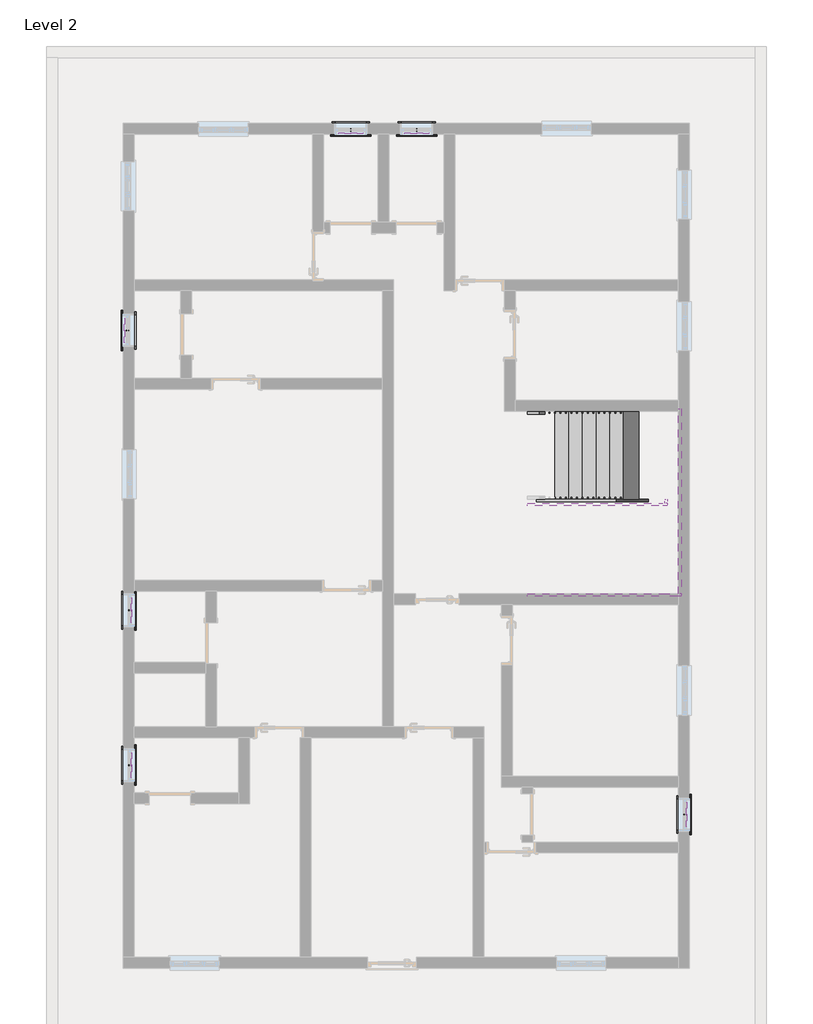
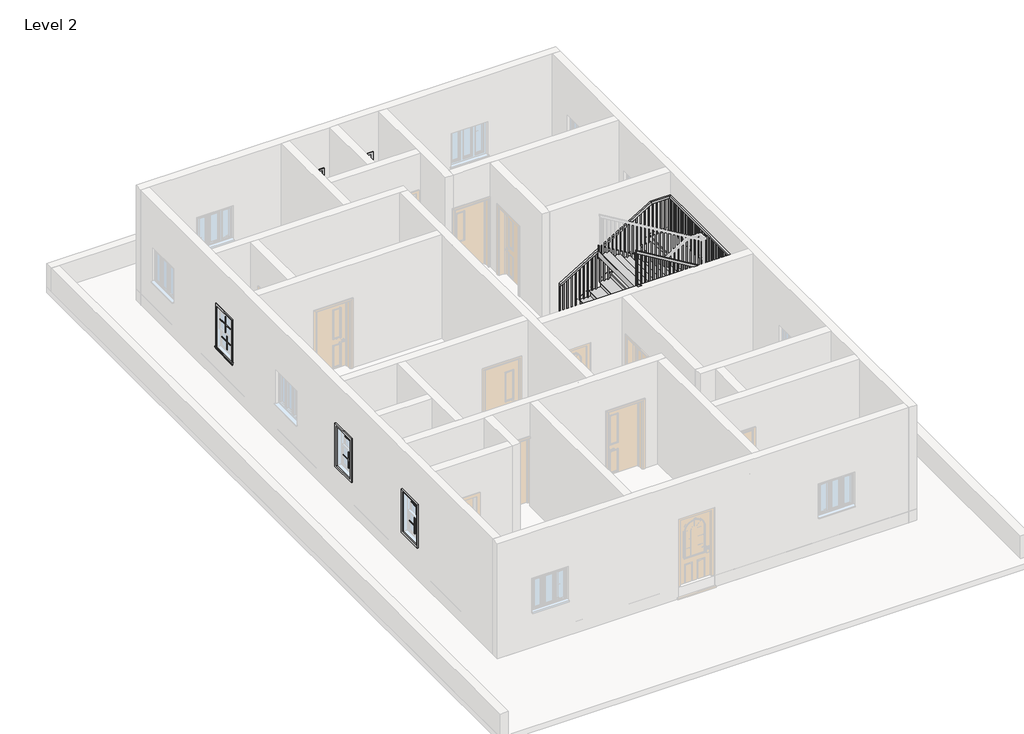
# One storey, part 3 of 3: 24 proxies, 6 members, 1 railing, 1 stair flight.
"""IFC4 building model written with IfcOpenShell, lengths in millimetres."""

from ifc_helpers import new_model, si_unit, frame, origin, place, context, project, spatial, polyline, outline, extrude, faceted_brep, transform, mapped, element, save
from components import muntin_pattern_2x2_muntin_pattern_2x2_eba6c5fb, trim_window_exterior_flat_with_sill_278e6a94, trim_window_interior_flat_picture_frame_e9fd5f45, stair_flight_de280899

model = new_model("IFC4")

# Units and contexts
model_context = context("Model", 3, world=origin())
ifc_project = project(units=[si_unit("LENGTHUNIT", "METRE", prefix="MILLI")], contexts=[model_context])

# Site, building, storey
site = spatial("IfcSite", under=ifc_project)
building = spatial("IfcBuilding", under=site)
storey = spatial("IfcBuildingStorey", under=building, Name="Level 2", Elevation=3048.0)

# Proxies
placement = place(None, origin())
muntin_pattern_2x2_muntin_pattern_2x2_shape = muntin_pattern_2x2_muntin_pattern_2x2_eba6c5fb(model_context)
element("IfcBuildingElementProxy", 1, Name="Muntin Pattern_2x2 : Muntin Pattern_2x2", ObjectType="Muntin Pattern_2x2 : Muntin Pattern_2x2", at=placement, inside=storey, context=model_context, shape_type="MappedRepresentation", body=[
    mapped(muntin_pattern_2x2_muntin_pattern_2x2_shape, transform((-13738.8961241, 8049.5344295, 4518.025), x_axis=(0.0, -1.0, 0.0), y_axis=(1.0, 0.0, 0.0), z_axis=(0.0, 0.0, 1.0))),
])
element("IfcBuildingElementProxy", 2, Name="Muntin Pattern_2x2 : Muntin Pattern_2x2", ObjectType="Muntin Pattern_2x2 : Muntin Pattern_2x2", at=placement, inside=storey, context=model_context, shape_type="MappedRepresentation", body=[
    mapped(muntin_pattern_2x2_muntin_pattern_2x2_shape, transform((-13783.3461241, 8049.5344295, 4038.6), x_axis=(0.0, -1.0, 0.0), y_axis=(1.0, 0.0, 0.0), z_axis=(0.0, 0.0, 1.0))),
])
element("IfcBuildingElementProxy", 3, Name="Muntin Pattern_2x2 : Muntin Pattern_2x2", ObjectType="Muntin Pattern_2x2 : Muntin Pattern_2x2", at=placement, inside=storey, context=model_context, shape_type="MappedRepresentation", body=[
    mapped(muntin_pattern_2x2_muntin_pattern_2x2_shape, transform((-13738.8961241, 5179.3344295, 4518.025), x_axis=(0.0, -1.0, 0.0), y_axis=(1.0, 0.0, 0.0), z_axis=(0.0, 0.0, 1.0))),
])
element("IfcBuildingElementProxy", 4, Name="Muntin Pattern_2x2 : Muntin Pattern_2x2", ObjectType="Muntin Pattern_2x2 : Muntin Pattern_2x2", at=placement, inside=storey, context=model_context, shape_type="MappedRepresentation", body=[
    mapped(muntin_pattern_2x2_muntin_pattern_2x2_shape, transform((-13783.3461241, 5179.3344295, 4038.6), x_axis=(0.0, -1.0, 0.0), y_axis=(1.0, 0.0, 0.0), z_axis=(0.0, 0.0, 1.0))),
])
element("IfcBuildingElementProxy", 5, Name="Muntin Pattern_2x2 : Muntin Pattern_2x2", ObjectType="Muntin Pattern_2x2 : Muntin Pattern_2x2", at=placement, inside=storey, context=model_context, shape_type="MappedRepresentation", body=[
    mapped(muntin_pattern_2x2_muntin_pattern_2x2_shape, transform((-13872.2461241, 13231.1344295, 4518.025), x_axis=(0.0, 1.0, 0.0), y_axis=(-1.0, 0.0, 0.0), z_axis=(0.0, 0.0, 1.0))),
])
element("IfcBuildingElementProxy", 6, Name="Muntin Pattern_2x2 : Muntin Pattern_2x2", ObjectType="Muntin Pattern_2x2 : Muntin Pattern_2x2", at=placement, inside=storey, context=model_context, shape_type="MappedRepresentation", body=[
    mapped(muntin_pattern_2x2_muntin_pattern_2x2_shape, transform((-13827.7961241, 13231.1344295, 4038.6), x_axis=(0.0, 1.0, 0.0), y_axis=(-1.0, 0.0, 0.0), z_axis=(0.0, 0.0, 1.0))),
])
element("IfcBuildingElementProxy", 7, Name="Muntin Pattern_2x2 : Muntin Pattern_2x2", ObjectType="Muntin Pattern_2x2 : Muntin Pattern_2x2", at=placement, inside=storey, context=model_context, shape_type="MappedRepresentation", body=[
    mapped(muntin_pattern_2x2_muntin_pattern_2x2_shape, transform((-9690.7711241, 16898.2594295, 4518.025), x_axis=(-1.0, 0.0, 0.0), y_axis=(0.0, -1.0, 0.0), z_axis=(0.0, 0.0, 1.0))),
])
element("IfcBuildingElementProxy", 8, Name="Muntin Pattern_2x2 : Muntin Pattern_2x2", ObjectType="Muntin Pattern_2x2 : Muntin Pattern_2x2", at=placement, inside=storey, context=model_context, shape_type="MappedRepresentation", body=[
    mapped(muntin_pattern_2x2_muntin_pattern_2x2_shape, transform((-9690.7711241, 16942.7094295, 4038.6), x_axis=(-1.0, 0.0, 0.0), y_axis=(0.0, -1.0, 0.0), z_axis=(0.0, 0.0, 1.0))),
])
element("IfcBuildingElementProxy", 9, Name="Muntin Pattern_2x2 : Muntin Pattern_2x2", ObjectType="Muntin Pattern_2x2 : Muntin Pattern_2x2", at=placement, inside=storey, context=model_context, shape_type="MappedRepresentation", body=[
    mapped(muntin_pattern_2x2_muntin_pattern_2x2_shape, transform((-8471.5711241, 16898.2594295, 4518.025), x_axis=(-1.0, 0.0, 0.0), y_axis=(0.0, -1.0, 0.0), z_axis=(0.0, 0.0, 1.0))),
])
element("IfcBuildingElementProxy", 10, Name="Muntin Pattern_2x2 : Muntin Pattern_2x2", ObjectType="Muntin Pattern_2x2 : Muntin Pattern_2x2", at=placement, inside=storey, context=model_context, shape_type="MappedRepresentation", body=[
    mapped(muntin_pattern_2x2_muntin_pattern_2x2_shape, transform((-8471.5711241, 16942.7094295, 4038.6), x_axis=(-1.0, 0.0, 0.0), y_axis=(0.0, -1.0, 0.0), z_axis=(0.0, 0.0, 1.0))),
])
element("IfcBuildingElementProxy", 11, Name="Muntin Pattern_2x2 : Muntin Pattern_2x2", ObjectType="Muntin Pattern_2x2 : Muntin Pattern_2x2", at=placement, inside=storey, context=model_context, shape_type="MappedRepresentation", body=[
    mapped(muntin_pattern_2x2_muntin_pattern_2x2_shape, transform((-3451.8961241, 4264.9344295, 4518.025), x_axis=(0.0, -1.0, 0.0), y_axis=(1.0, 0.0, 0.0), z_axis=(0.0, 0.0, 1.0))),
])
element("IfcBuildingElementProxy", 12, Name="Muntin Pattern_2x2 : Muntin Pattern_2x2", ObjectType="Muntin Pattern_2x2 : Muntin Pattern_2x2", at=placement, inside=storey, context=model_context, shape_type="MappedRepresentation", body=[
    mapped(muntin_pattern_2x2_muntin_pattern_2x2_shape, transform((-3496.3461241, 4264.9344295, 4038.6), x_axis=(0.0, -1.0, 0.0), y_axis=(1.0, 0.0, 0.0), z_axis=(0.0, 0.0, 1.0))),
])
trim_window_exterior_flat_with_sill_shape = trim_window_exterior_flat_with_sill_278e6a94(model_context)
element("IfcBuildingElementProxy", 13, Name="Trim-Window-Exterior-Flat : with Sill", ObjectType="Trim-Window-Exterior-Flat : with Sill", at=placement, inside=storey, context=model_context, shape_type="MappedRepresentation", body=[
    mapped(trim_window_exterior_flat_with_sill_shape, transform((-13703.9711241, 8049.5344295, 5029.2), x_axis=(0.0, 1.0, 0.0), y_axis=(0.0, 0.0, 1.0), z_axis=(1.0, 0.0, 0.0))),
])
element("IfcBuildingElementProxy", 14, Name="Trim-Window-Exterior-Flat : with Sill", ObjectType="Trim-Window-Exterior-Flat : with Sill", at=placement, inside=storey, context=model_context, shape_type="MappedRepresentation", body=[
    mapped(trim_window_exterior_flat_with_sill_shape, transform((-13703.9711241, 5179.3344295, 5029.2), x_axis=(0.0, 1.0, 0.0), y_axis=(0.0, 0.0, 1.0), z_axis=(1.0, 0.0, 0.0))),
])
element("IfcBuildingElementProxy", 15, Name="Trim-Window-Exterior-Flat : with Sill", ObjectType="Trim-Window-Exterior-Flat : with Sill", at=placement, inside=storey, context=model_context, shape_type="MappedRepresentation", body=[
    mapped(trim_window_exterior_flat_with_sill_shape, transform((-13907.1711241, 13231.1344295, 5029.2), x_axis=(0.0, -1.0, 0.0), y_axis=(0.0, 0.0, 1.0), z_axis=(-1.0, 0.0, 0.0))),
])
element("IfcBuildingElementProxy", 16, Name="Trim-Window-Exterior-Flat : with Sill", ObjectType="Trim-Window-Exterior-Flat : with Sill", at=placement, inside=storey, context=model_context, shape_type="MappedRepresentation", body=[
    mapped(trim_window_exterior_flat_with_sill_shape, transform((-9690.7711241, 16863.3344295, 5029.2), x_axis=(1.0, 0.0, 0.0), y_axis=(0.0, 0.0, 1.0), z_axis=(0.0, -1.0, 0.0))),
])
element("IfcBuildingElementProxy", 17, Name="Trim-Window-Exterior-Flat : with Sill", ObjectType="Trim-Window-Exterior-Flat : with Sill", at=placement, inside=storey, context=model_context, shape_type="MappedRepresentation", body=[
    mapped(trim_window_exterior_flat_with_sill_shape, transform((-8471.5711241, 16863.3344295, 5029.2), x_axis=(1.0, 0.0, 0.0), y_axis=(0.0, 0.0, 1.0), z_axis=(0.0, -1.0, 0.0))),
])
element("IfcBuildingElementProxy", 18, Name="Trim-Window-Exterior-Flat : with Sill", ObjectType="Trim-Window-Exterior-Flat : with Sill", at=placement, inside=storey, context=model_context, shape_type="MappedRepresentation", body=[
    mapped(trim_window_exterior_flat_with_sill_shape, transform((-3416.9711241, 4264.9344295, 5029.2), x_axis=(0.0, 1.0, 0.0), y_axis=(0.0, 0.0, 1.0), z_axis=(1.0, 0.0, 0.0))),
])
trim_window_interior_flat_picture_frame_shape = trim_window_interior_flat_picture_frame_e9fd5f45(model_context)
element("IfcBuildingElementProxy", 19, Name="Trim-Window-Interior-Flat : Picture Frame", ObjectType="Trim-Window-Interior-Flat : Picture Frame", at=placement, inside=storey, context=model_context, shape_type="MappedRepresentation", body=[
    mapped(trim_window_interior_flat_picture_frame_shape, transform((-13907.1711241, 8049.5344295, 5029.2), x_axis=(0.0, -1.0, 0.0), y_axis=(0.0, 0.0, 1.0), z_axis=(-1.0, 0.0, 0.0))),
])
element("IfcBuildingElementProxy", 20, Name="Trim-Window-Interior-Flat : Picture Frame", ObjectType="Trim-Window-Interior-Flat : Picture Frame", at=placement, inside=storey, context=model_context, shape_type="MappedRepresentation", body=[
    mapped(trim_window_interior_flat_picture_frame_shape, transform((-13907.1711241, 5179.3344295, 5029.2), x_axis=(0.0, -1.0, 0.0), y_axis=(0.0, 0.0, 1.0), z_axis=(-1.0, 0.0, 0.0))),
])
element("IfcBuildingElementProxy", 21, Name="Trim-Window-Interior-Flat : Picture Frame", ObjectType="Trim-Window-Interior-Flat : Picture Frame", at=placement, inside=storey, context=model_context, shape_type="MappedRepresentation", body=[
    mapped(trim_window_interior_flat_picture_frame_shape, transform((-13703.9711241, 13231.1344295, 5029.2), x_axis=(0.0, 1.0, 0.0), y_axis=(0.0, 0.0, 1.0), z_axis=(1.0, 0.0, 0.0))),
])
element("IfcBuildingElementProxy", 22, Name="Trim-Window-Interior-Flat : Picture Frame", ObjectType="Trim-Window-Interior-Flat : Picture Frame", at=placement, inside=storey, context=model_context, shape_type="MappedRepresentation", body=[
    mapped(trim_window_interior_flat_picture_frame_shape, transform((-9690.7711241, 17066.5344295, 5029.2), x_axis=(-1.0, 0.0, 0.0), y_axis=(0.0, 0.0, 1.0), z_axis=(0.0, 1.0, 0.0))),
])
element("IfcBuildingElementProxy", 23, Name="Trim-Window-Interior-Flat : Picture Frame", ObjectType="Trim-Window-Interior-Flat : Picture Frame", at=placement, inside=storey, context=model_context, shape_type="MappedRepresentation", body=[
    mapped(trim_window_interior_flat_picture_frame_shape, transform((-8471.5711241, 17066.5344295, 5029.2), x_axis=(-1.0, 0.0, 0.0), y_axis=(0.0, 0.0, 1.0), z_axis=(0.0, 1.0, 0.0))),
])
element("IfcBuildingElementProxy", 24, Name="Trim-Window-Interior-Flat : Picture Frame", ObjectType="Trim-Window-Interior-Flat : Picture Frame", at=placement, inside=storey, context=model_context, shape_type="MappedRepresentation", body=[
    mapped(trim_window_interior_flat_picture_frame_shape, transform((-3620.1711241, 4264.9344295, 5029.2), x_axis=(0.0, -1.0, 0.0), y_axis=(0.0, 0.0, 1.0), z_axis=(-1.0, 0.0, 0.0))),
])

# Members
element("IfcMember", 25, ObjectType="Stringer - 2\" Width", at=placement, inside=storey, context=model_context, shape_type="SweptSolid", body=[
    extrude(outline(polyline([(3259.5517384, -6414.1711241), (3048.0, -6414.1711241), (3048.0, -6174.3326423), (4580.4969109, -3620.1711241), (4648.2, -3620.1711241), (4648.2, -4099.7573548), (3259.5517384, -6414.1711241)])), frame((0.0, 11732.5344295, 0.0), z_axis=(0.0, 1.0, 0.0), x_axis=(0.0, 0.0, 1.0)), (0.0, 0.0, 1.0), 50.8),
])
element("IfcMember", 26, ObjectType="Stringer - 2\" Width", at=placement, inside=storey, context=model_context, shape_type="SweptSolid", body=[
    extrude(outline(polyline([(-3620.1711241, 11783.3344295), (-3569.3711241, 11783.3344295), (-3569.3711241, 8354.3344295), (-3620.1711241, 8354.3344295), (-3620.1711241, 11783.3344295)])), frame((0.0, 0.0, 4343.4), z_axis=(0.0, 0.0, 1.0), x_axis=(1.0, 0.0, 0.0)), (0.0, 0.0, 1.0), 304.8),
])
element("IfcMember", 27, ObjectType="Stringer - 2\" Width", at=placement, inside=storey, context=model_context, shape_type="SweptSolid", body=[
    extrude(outline(polyline([(4343.4, -3569.3711241), (4448.2717384, -3569.3711241), (6155.1517384, -6414.1711241), (5799.6969109, -6414.1711241), (4343.4, -3987.0096058), (4343.4, -3569.3711241)])), frame((0.0, 8303.5344295, 0.0), z_axis=(0.0, 1.0, 0.0), x_axis=(0.0, 0.0, 1.0)), (0.0, 0.0, 1.0), 50.8),
])
element("IfcMember", 28, ObjectType="Stringer - 2\" Width", at=placement, inside=storey, context=model_context, shape_type="SweptSolid", body=[
    extrude(outline(polyline([(3259.5517384, -6414.1711241), (3048.0, -6414.1711241), (3048.0, -6174.3326423), (4428.0969109, -3874.1711241), (4648.2, -3874.1711241), (4648.2, -4099.7573548), (3259.5517384, -6414.1711241)])), frame((0.0, 10056.1344295, 0.0), z_axis=(0.0, 1.0, 0.0), x_axis=(0.0, 0.0, 1.0)), (0.0, 0.0, 1.0), 50.8),
])
element("IfcMember", 29, ObjectType="Stringer - 2\" Width", at=placement, inside=storey, context=model_context, shape_type="SweptSolid", body=[
    extrude(outline(polyline([(-3874.1711241, 10106.9344295), (-3823.3711241, 10106.9344295), (-3823.3711241, 10030.7344295), (-3874.1711241, 10030.7344295), (-3874.1711241, 10106.9344295)])), frame((0.0, 0.0, 4343.4), z_axis=(0.0, 0.0, 1.0), x_axis=(1.0, 0.0, 0.0)), (0.0, 0.0, 1.0), 304.8),
])
element("IfcMember", 30, ObjectType="Stringer - 2\" Width", at=placement, inside=storey, context=model_context, shape_type="SweptSolid", body=[
    extrude(outline(polyline([(4343.4, -3823.3711241), (4600.6717384, -3823.3711241), (6155.1517384, -6414.1711241), (5799.6969109, -6414.1711241), (4343.4, -3987.0096058), (4343.4, -3823.3711241)])), frame((0.0, 9979.9344295, 0.0), z_axis=(0.0, 1.0, 0.0), x_axis=(0.0, 0.0, 1.0)), (0.0, 0.0, 1.0), 50.8),
])

# Railing
element("IfcRailing", 31, ObjectType="Handrail - Rectangular", at=placement, inside=storey, context=model_context, shape_type="SolidModel", body=[
    faceted_brep([(-6414.1711241, 11732.5344295, 4114.8), (-6414.1711241, 11732.5344295, 4055.5575287), (-6414.1711241, 11681.7344295, 4055.5575287), (-6414.1711241, 11681.7344295, 4114.8), (-4128.1711241, 11732.5344295, 5486.4), (-4114.1003386, 11732.5344295, 5435.6), (-4114.1003386, 11681.7344295, 5435.6), (-4128.1711241, 11681.7344295, 5486.4), (-3620.1711241, 11732.5344295, 5486.4), (-3620.1711241, 11732.5344295, 5435.6), (-3670.9711241, 11681.7344295, 5435.6), (-3670.9711241, 11681.7344295, 5486.4), (-3620.1711241, 8354.3344295, 5486.4), (-3620.1711241, 8354.3344295, 5435.6), (-3670.9711241, 8405.1344295, 5435.6), (-3670.9711241, 8405.1344295, 5486.4), (-3874.1711241, 8354.3344295, 5486.4), (-3888.2419095, 8354.3344295, 5435.6), (-3888.2419095, 8405.1344295, 5435.6), (-3874.1711241, 8405.1344295, 5486.4), (-6414.1711241, 8354.3344295, 7010.4), (-6414.1711241, 8405.1344295, 7010.4), (-6414.1711241, 8405.1344295, 6951.1575287), (-6414.1711241, 8354.3344295, 6951.1575287)], [[[0, 1, 2, 3]], [[1, 0, 4, 5]], [[2, 1, 5, 6]], [[3, 2, 6, 7]], [[0, 3, 7, 4]], [[5, 4, 8, 9]], [[6, 5, 9, 10]], [[7, 6, 10, 11]], [[4, 7, 11, 8]], [[9, 8, 12, 13]], [[10, 9, 13, 14]], [[11, 10, 14, 15]], [[8, 11, 15, 12]], [[13, 12, 16, 17]], [[14, 13, 17, 18]], [[15, 14, 18, 19]], [[12, 15, 19, 16]], [[20, 21, 22, 23]], [[17, 16, 20, 23]], [[18, 17, 23, 22]], [[19, 18, 22, 21]], [[16, 19, 21, 20]]]),
    extrude(outline(polyline([(6941.6325287, -6398.2961241), (5943.6, -6398.2961241), (5943.6, -6379.2461241), (6930.2025287, -6379.2461241), (6941.6325287, -6398.2961241)])), frame((0.0, 8370.2094295, 0.0), z_axis=(0.0, 1.0, 0.0), x_axis=(0.0, 0.0, 1.0)), (0.0, 0.0, 1.0), 19.05),
    extrude(outline(polyline([(6880.6725287, -6296.6961241), (5943.6, -6296.6961241), (5943.6, -6277.6461241), (6869.2425287, -6277.6461241), (6880.6725287, -6296.6961241)])), frame((0.0, 8370.2094295, 0.0), z_axis=(0.0, 1.0, 0.0), x_axis=(0.0, 0.0, 1.0)), (0.0, 0.0, 1.0), 19.05),
    extrude(outline(polyline([(6819.7125287, -6195.0961241), (5943.6, -6195.0961241), (5943.6, -6176.0461241), (6808.2825287, -6176.0461241), (6819.7125287, -6195.0961241)])), frame((0.0, 8370.2094295, 0.0), z_axis=(0.0, 1.0, 0.0), x_axis=(0.0, 0.0, 1.0)), (0.0, 0.0, 1.0), 19.05),
    extrude(outline(polyline([(6758.7525287, -6093.4961241), (5791.2, -6093.4961241), (5791.2, -6074.4461241), (6747.3225287, -6074.4461241), (6758.7525287, -6093.4961241)])), frame((0.0, 8370.2094295, 0.0), z_axis=(0.0, 1.0, 0.0), x_axis=(0.0, 0.0, 1.0)), (0.0, 0.0, 1.0), 19.05),
    extrude(outline(polyline([(6697.7925287, -5991.8961241), (5791.2, -5991.8961241), (5791.2, -5972.8461241), (6686.3625287, -5972.8461241), (6697.7925287, -5991.8961241)])), frame((0.0, 8370.2094295, 0.0), z_axis=(0.0, 1.0, 0.0), x_axis=(0.0, 0.0, 1.0)), (0.0, 0.0, 1.0), 19.05),
    extrude(outline(polyline([(6636.8325287, -5890.2961241), (5638.8, -5890.2961241), (5638.8, -5871.2461241), (6625.4025287, -5871.2461241), (6636.8325287, -5890.2961241)])), frame((0.0, 8370.2094295, 0.0), z_axis=(0.0, 1.0, 0.0), x_axis=(0.0, 0.0, 1.0)), (0.0, 0.0, 1.0), 19.05),
    extrude(outline(polyline([(6575.8725287, -5788.6961241), (5638.8, -5788.6961241), (5638.8, -5769.6461241), (6564.4425287, -5769.6461241), (6575.8725287, -5788.6961241)])), frame((0.0, 8370.2094295, 0.0), z_axis=(0.0, 1.0, 0.0), x_axis=(0.0, 0.0, 1.0)), (0.0, 0.0, 1.0), 19.05),
    extrude(outline(polyline([(6514.9125287, -5687.0961241), (5638.8, -5687.0961241), (5638.8, -5668.0461241), (6503.4825287, -5668.0461241), (6514.9125287, -5687.0961241)])), frame((0.0, 8370.2094295, 0.0), z_axis=(0.0, 1.0, 0.0), x_axis=(0.0, 0.0, 1.0)), (0.0, 0.0, 1.0), 19.05),
    extrude(outline(polyline([(6453.9525287, -5585.4961241), (5486.4, -5585.4961241), (5486.4, -5566.4461241), (6442.5225287, -5566.4461241), (6453.9525287, -5585.4961241)])), frame((0.0, 8370.2094295, 0.0), z_axis=(0.0, 1.0, 0.0), x_axis=(0.0, 0.0, 1.0)), (0.0, 0.0, 1.0), 19.05),
    extrude(outline(polyline([(6392.9925287, -5483.8961241), (5486.4, -5483.8961241), (5486.4, -5464.8461241), (6381.5625287, -5464.8461241), (6392.9925287, -5483.8961241)])), frame((0.0, 8370.2094295, 0.0), z_axis=(0.0, 1.0, 0.0), x_axis=(0.0, 0.0, 1.0)), (0.0, 0.0, 1.0), 19.05),
    extrude(outline(polyline([(6332.0325287, -5382.2961241), (5334.0, -5382.2961241), (5334.0, -5363.2461241), (6320.6025287, -5363.2461241), (6332.0325287, -5382.2961241)])), frame((0.0, 8370.2094295, 0.0), z_axis=(0.0, 1.0, 0.0), x_axis=(0.0, 0.0, 1.0)), (0.0, 0.0, 1.0), 19.05),
    extrude(outline(polyline([(6271.0725287, -5280.6961241), (5334.0, -5280.6961241), (5334.0, -5261.6461241), (6259.6425287, -5261.6461241), (6271.0725287, -5280.6961241)])), frame((0.0, 8370.2094295, 0.0), z_axis=(0.0, 1.0, 0.0), x_axis=(0.0, 0.0, 1.0)), (0.0, 0.0, 1.0), 19.05),
    extrude(outline(polyline([(6210.1125287, -5179.0961241), (5334.0, -5179.0961241), (5334.0, -5160.0461241), (6198.6825287, -5160.0461241), (6210.1125287, -5179.0961241)])), frame((0.0, 8370.2094295, 0.0), z_axis=(0.0, 1.0, 0.0), x_axis=(0.0, 0.0, 1.0)), (0.0, 0.0, 1.0), 19.05),
    extrude(outline(polyline([(6149.1525287, -5077.4961241), (5181.6, -5077.4961241), (5181.6, -5058.4461241), (6137.7225287, -5058.4461241), (6149.1525287, -5077.4961241)])), frame((0.0, 8370.2094295, 0.0), z_axis=(0.0, 1.0, 0.0), x_axis=(0.0, 0.0, 1.0)), (0.0, 0.0, 1.0), 19.05),
    extrude(outline(polyline([(6088.1925287, -4975.8961241), (5181.6, -4975.8961241), (5181.6, -4956.8461241), (6076.7625287, -4956.8461241), (6088.1925287, -4975.8961241)])), frame((0.0, 8370.2094295, 0.0), z_axis=(0.0, 1.0, 0.0), x_axis=(0.0, 0.0, 1.0)), (0.0, 0.0, 1.0), 19.05),
    extrude(outline(polyline([(6027.2325287, -4874.2961241), (5029.2, -4874.2961241), (5029.2, -4855.2461241), (6015.8025287, -4855.2461241), (6027.2325287, -4874.2961241)])), frame((0.0, 8370.2094295, 0.0), z_axis=(0.0, 1.0, 0.0), x_axis=(0.0, 0.0, 1.0)), (0.0, 0.0, 1.0), 19.05),
    extrude(outline(polyline([(5966.2725287, -4772.6961241), (5029.2, -4772.6961241), (5029.2, -4753.6461241), (5954.8425287, -4753.6461241), (5966.2725287, -4772.6961241)])), frame((0.0, 8370.2094295, 0.0), z_axis=(0.0, 1.0, 0.0), x_axis=(0.0, 0.0, 1.0)), (0.0, 0.0, 1.0), 19.05),
    extrude(outline(polyline([(5905.3125287, -4671.0961241), (5029.2, -4671.0961241), (5029.2, -4652.0461241), (5893.8825287, -4652.0461241), (5905.3125287, -4671.0961241)])), frame((0.0, 8370.2094295, 0.0), z_axis=(0.0, 1.0, 0.0), x_axis=(0.0, 0.0, 1.0)), (0.0, 0.0, 1.0), 19.05),
    extrude(outline(polyline([(5844.3525287, -4569.4961241), (4876.8, -4569.4961241), (4876.8, -4550.4461241), (5832.9225287, -4550.4461241), (5844.3525287, -4569.4961241)])), frame((0.0, 8370.2094295, 0.0), z_axis=(0.0, 1.0, 0.0), x_axis=(0.0, 0.0, 1.0)), (0.0, 0.0, 1.0), 19.05),
    extrude(outline(polyline([(5783.3925287, -4467.8961241), (4876.8, -4467.8961241), (4876.8, -4448.8461241), (5771.9625287, -4448.8461241), (5783.3925287, -4467.8961241)])), frame((0.0, 8370.2094295, 0.0), z_axis=(0.0, 1.0, 0.0), x_axis=(0.0, 0.0, 1.0)), (0.0, 0.0, 1.0), 19.05),
    extrude(outline(polyline([(5722.4325287, -4366.2961241), (4724.4, -4366.2961241), (4724.4, -4347.2461241), (5711.0025287, -4347.2461241), (5722.4325287, -4366.2961241)])), frame((0.0, 8370.2094295, 0.0), z_axis=(0.0, 1.0, 0.0), x_axis=(0.0, 0.0, 1.0)), (0.0, 0.0, 1.0), 19.05),
    extrude(outline(polyline([(5661.4725287, -4264.6961241), (4724.4, -4264.6961241), (4724.4, -4245.6461241), (5650.0425287, -4245.6461241), (5661.4725287, -4264.6961241)])), frame((0.0, 8370.2094295, 0.0), z_axis=(0.0, 1.0, 0.0), x_axis=(0.0, 0.0, 1.0)), (0.0, 0.0, 1.0), 19.05),
    extrude(outline(polyline([(5600.5125287, -4163.0961241), (4724.4, -4163.0961241), (4724.4, -4144.0461241), (5589.0825287, -4144.0461241), (5600.5125287, -4163.0961241)])), frame((0.0, 8370.2094295, 0.0), z_axis=(0.0, 1.0, 0.0), x_axis=(0.0, 0.0, 1.0)), (0.0, 0.0, 1.0), 19.05),
    extrude(outline(polyline([(5539.5525287, -4061.4961241), (4572.0, -4061.4961241), (4572.0, -4042.4461241), (5528.1225287, -4042.4461241), (5539.5525287, -4061.4961241)])), frame((0.0, 8370.2094295, 0.0), z_axis=(0.0, 1.0, 0.0), x_axis=(0.0, 0.0, 1.0)), (0.0, 0.0, 1.0), 19.05),
    extrude(outline(polyline([(5478.5925287, -3959.8961241), (4572.0, -3959.8961241), (4572.0, -3940.8461241), (5467.1625287, -3940.8461241), (5478.5925287, -3959.8961241)])), frame((0.0, 8370.2094295, 0.0), z_axis=(0.0, 1.0, 0.0), x_axis=(0.0, 0.0, 1.0)), (0.0, 0.0, 1.0), 19.05),
    extrude(outline(polyline([(-3839.2461241, 8370.2094295), (-3858.2961241, 8370.2094295), (-3858.2961241, 8389.2594295), (-3839.2461241, 8389.2594295), (-3839.2461241, 8370.2094295)])), frame((0.0, 0.0, 4572.0), z_axis=(0.0, 0.0, 1.0), x_axis=(1.0, 0.0, 0.0)), (0.0, 0.0, 1.0), 863.6),
    extrude(outline(polyline([(-3737.6461241, 8370.2094295), (-3756.6961241, 8370.2094295), (-3756.6961241, 8389.2594295), (-3737.6461241, 8389.2594295), (-3737.6461241, 8370.2094295)])), frame((0.0, 0.0, 4572.0), z_axis=(0.0, 0.0, 1.0), x_axis=(1.0, 0.0, 0.0)), (0.0, 0.0, 1.0), 863.6),
    extrude(outline(polyline([(-3636.0461241, 8465.4594295), (-3636.0461241, 8446.4094295), (-3655.0961241, 8446.4094295), (-3655.0961241, 8465.4594295), (-3636.0461241, 8465.4594295)])), frame((0.0, 0.0, 4572.0), z_axis=(0.0, 0.0, 1.0), x_axis=(1.0, 0.0, 0.0)), (0.0, 0.0, 1.0), 863.6),
    extrude(outline(polyline([(-3636.0461241, 8567.0594295), (-3636.0461241, 8548.0094295), (-3655.0961241, 8548.0094295), (-3655.0961241, 8567.0594295), (-3636.0461241, 8567.0594295)])), frame((0.0, 0.0, 4572.0), z_axis=(0.0, 0.0, 1.0), x_axis=(1.0, 0.0, 0.0)), (0.0, 0.0, 1.0), 863.6),
    extrude(outline(polyline([(-3636.0461241, 8668.6594295), (-3636.0461241, 8649.6094295), (-3655.0961241, 8649.6094295), (-3655.0961241, 8668.6594295), (-3636.0461241, 8668.6594295)])), frame((0.0, 0.0, 4572.0), z_axis=(0.0, 0.0, 1.0), x_axis=(1.0, 0.0, 0.0)), (0.0, 0.0, 1.0), 863.6),
    extrude(outline(polyline([(-3636.0461241, 8770.2594295), (-3636.0461241, 8751.2094295), (-3655.0961241, 8751.2094295), (-3655.0961241, 8770.2594295), (-3636.0461241, 8770.2594295)])), frame((0.0, 0.0, 4572.0), z_axis=(0.0, 0.0, 1.0), x_axis=(1.0, 0.0, 0.0)), (0.0, 0.0, 1.0), 863.6),
    extrude(outline(polyline([(-3636.0461241, 8871.8594295), (-3636.0461241, 8852.8094295), (-3655.0961241, 8852.8094295), (-3655.0961241, 8871.8594295), (-3636.0461241, 8871.8594295)])), frame((0.0, 0.0, 4572.0), z_axis=(0.0, 0.0, 1.0), x_axis=(1.0, 0.0, 0.0)), (0.0, 0.0, 1.0), 863.6),
    extrude(outline(polyline([(-3636.0461241, 8973.4594295), (-3636.0461241, 8954.4094295), (-3655.0961241, 8954.4094295), (-3655.0961241, 8973.4594295), (-3636.0461241, 8973.4594295)])), frame((0.0, 0.0, 4572.0), z_axis=(0.0, 0.0, 1.0), x_axis=(1.0, 0.0, 0.0)), (0.0, 0.0, 1.0), 863.6),
    extrude(outline(polyline([(-3636.0461241, 9075.0594295), (-3636.0461241, 9056.0094295), (-3655.0961241, 9056.0094295), (-3655.0961241, 9075.0594295), (-3636.0461241, 9075.0594295)])), frame((0.0, 0.0, 4572.0), z_axis=(0.0, 0.0, 1.0), x_axis=(1.0, 0.0, 0.0)), (0.0, 0.0, 1.0), 863.6),
    extrude(outline(polyline([(-3636.0461241, 9176.6594295), (-3636.0461241, 9157.6094295), (-3655.0961241, 9157.6094295), (-3655.0961241, 9176.6594295), (-3636.0461241, 9176.6594295)])), frame((0.0, 0.0, 4572.0), z_axis=(0.0, 0.0, 1.0), x_axis=(1.0, 0.0, 0.0)), (0.0, 0.0, 1.0), 863.6),
    extrude(outline(polyline([(-3636.0461241, 9278.2594295), (-3636.0461241, 9259.2094295), (-3655.0961241, 9259.2094295), (-3655.0961241, 9278.2594295), (-3636.0461241, 9278.2594295)])), frame((0.0, 0.0, 4572.0), z_axis=(0.0, 0.0, 1.0), x_axis=(1.0, 0.0, 0.0)), (0.0, 0.0, 1.0), 863.6),
    extrude(outline(polyline([(-3636.0461241, 9379.8594295), (-3636.0461241, 9360.8094295), (-3655.0961241, 9360.8094295), (-3655.0961241, 9379.8594295), (-3636.0461241, 9379.8594295)])), frame((0.0, 0.0, 4572.0), z_axis=(0.0, 0.0, 1.0), x_axis=(1.0, 0.0, 0.0)), (0.0, 0.0, 1.0), 863.6),
    extrude(outline(polyline([(-3636.0461241, 9481.4594295), (-3636.0461241, 9462.4094295), (-3655.0961241, 9462.4094295), (-3655.0961241, 9481.4594295), (-3636.0461241, 9481.4594295)])), frame((0.0, 0.0, 4572.0), z_axis=(0.0, 0.0, 1.0), x_axis=(1.0, 0.0, 0.0)), (0.0, 0.0, 1.0), 863.6),
    extrude(outline(polyline([(-3636.0461241, 9583.0594295), (-3636.0461241, 9564.0094295), (-3655.0961241, 9564.0094295), (-3655.0961241, 9583.0594295), (-3636.0461241, 9583.0594295)])), frame((0.0, 0.0, 4572.0), z_axis=(0.0, 0.0, 1.0), x_axis=(1.0, 0.0, 0.0)), (0.0, 0.0, 1.0), 863.6),
    extrude(outline(polyline([(-3636.0461241, 9684.6594295), (-3636.0461241, 9665.6094295), (-3655.0961241, 9665.6094295), (-3655.0961241, 9684.6594295), (-3636.0461241, 9684.6594295)])), frame((0.0, 0.0, 4572.0), z_axis=(0.0, 0.0, 1.0), x_axis=(1.0, 0.0, 0.0)), (0.0, 0.0, 1.0), 863.6),
    extrude(outline(polyline([(-3636.0461241, 9786.2594295), (-3636.0461241, 9767.2094295), (-3655.0961241, 9767.2094295), (-3655.0961241, 9786.2594295), (-3636.0461241, 9786.2594295)])), frame((0.0, 0.0, 4572.0), z_axis=(0.0, 0.0, 1.0), x_axis=(1.0, 0.0, 0.0)), (0.0, 0.0, 1.0), 863.6),
    extrude(outline(polyline([(-3636.0461241, 9887.8594295), (-3636.0461241, 9868.8094295), (-3655.0961241, 9868.8094295), (-3655.0961241, 9887.8594295), (-3636.0461241, 9887.8594295)])), frame((0.0, 0.0, 4572.0), z_axis=(0.0, 0.0, 1.0), x_axis=(1.0, 0.0, 0.0)), (0.0, 0.0, 1.0), 863.6),
    extrude(outline(polyline([(-3636.0461241, 9989.4594295), (-3636.0461241, 9970.4094295), (-3655.0961241, 9970.4094295), (-3655.0961241, 9989.4594295), (-3636.0461241, 9989.4594295)])), frame((0.0, 0.0, 4572.0), z_axis=(0.0, 0.0, 1.0), x_axis=(1.0, 0.0, 0.0)), (0.0, 0.0, 1.0), 863.6),
    extrude(outline(polyline([(-3636.0461241, 10091.0594295), (-3636.0461241, 10072.0094295), (-3655.0961241, 10072.0094295), (-3655.0961241, 10091.0594295), (-3636.0461241, 10091.0594295)])), frame((0.0, 0.0, 4572.0), z_axis=(0.0, 0.0, 1.0), x_axis=(1.0, 0.0, 0.0)), (0.0, 0.0, 1.0), 863.6),
    extrude(outline(polyline([(-3636.0461241, 10192.6594295), (-3636.0461241, 10173.6094295), (-3655.0961241, 10173.6094295), (-3655.0961241, 10192.6594295), (-3636.0461241, 10192.6594295)])), frame((0.0, 0.0, 4572.0), z_axis=(0.0, 0.0, 1.0), x_axis=(1.0, 0.0, 0.0)), (0.0, 0.0, 1.0), 863.6),
    extrude(outline(polyline([(-3636.0461241, 10294.2594295), (-3636.0461241, 10275.2094295), (-3655.0961241, 10275.2094295), (-3655.0961241, 10294.2594295), (-3636.0461241, 10294.2594295)])), frame((0.0, 0.0, 4572.0), z_axis=(0.0, 0.0, 1.0), x_axis=(1.0, 0.0, 0.0)), (0.0, 0.0, 1.0), 863.6),
    extrude(outline(polyline([(-3636.0461241, 10395.8594295), (-3636.0461241, 10376.8094295), (-3655.0961241, 10376.8094295), (-3655.0961241, 10395.8594295), (-3636.0461241, 10395.8594295)])), frame((0.0, 0.0, 4572.0), z_axis=(0.0, 0.0, 1.0), x_axis=(1.0, 0.0, 0.0)), (0.0, 0.0, 1.0), 863.6),
    extrude(outline(polyline([(-3636.0461241, 10497.4594295), (-3636.0461241, 10478.4094295), (-3655.0961241, 10478.4094295), (-3655.0961241, 10497.4594295), (-3636.0461241, 10497.4594295)])), frame((0.0, 0.0, 4572.0), z_axis=(0.0, 0.0, 1.0), x_axis=(1.0, 0.0, 0.0)), (0.0, 0.0, 1.0), 863.6),
    extrude(outline(polyline([(-3636.0461241, 10599.0594295), (-3636.0461241, 10580.0094295), (-3655.0961241, 10580.0094295), (-3655.0961241, 10599.0594295), (-3636.0461241, 10599.0594295)])), frame((0.0, 0.0, 4572.0), z_axis=(0.0, 0.0, 1.0), x_axis=(1.0, 0.0, 0.0)), (0.0, 0.0, 1.0), 863.6),
    extrude(outline(polyline([(-3636.0461241, 10700.6594295), (-3636.0461241, 10681.6094295), (-3655.0961241, 10681.6094295), (-3655.0961241, 10700.6594295), (-3636.0461241, 10700.6594295)])), frame((0.0, 0.0, 4572.0), z_axis=(0.0, 0.0, 1.0), x_axis=(1.0, 0.0, 0.0)), (0.0, 0.0, 1.0), 863.6),
    extrude(outline(polyline([(-3636.0461241, 10802.2594295), (-3636.0461241, 10783.2094295), (-3655.0961241, 10783.2094295), (-3655.0961241, 10802.2594295), (-3636.0461241, 10802.2594295)])), frame((0.0, 0.0, 4572.0), z_axis=(0.0, 0.0, 1.0), x_axis=(1.0, 0.0, 0.0)), (0.0, 0.0, 1.0), 863.6),
    extrude(outline(polyline([(-3636.0461241, 10903.8594295), (-3636.0461241, 10884.8094295), (-3655.0961241, 10884.8094295), (-3655.0961241, 10903.8594295), (-3636.0461241, 10903.8594295)])), frame((0.0, 0.0, 4572.0), z_axis=(0.0, 0.0, 1.0), x_axis=(1.0, 0.0, 0.0)), (0.0, 0.0, 1.0), 863.6),
    extrude(outline(polyline([(-3636.0461241, 11005.4594295), (-3636.0461241, 10986.4094295), (-3655.0961241, 10986.4094295), (-3655.0961241, 11005.4594295), (-3636.0461241, 11005.4594295)])), frame((0.0, 0.0, 4572.0), z_axis=(0.0, 0.0, 1.0), x_axis=(1.0, 0.0, 0.0)), (0.0, 0.0, 1.0), 863.6),
    extrude(outline(polyline([(-3636.0461241, 11107.0594295), (-3636.0461241, 11088.0094295), (-3655.0961241, 11088.0094295), (-3655.0961241, 11107.0594295), (-3636.0461241, 11107.0594295)])), frame((0.0, 0.0, 4572.0), z_axis=(0.0, 0.0, 1.0), x_axis=(1.0, 0.0, 0.0)), (0.0, 0.0, 1.0), 863.6),
    extrude(outline(polyline([(-3636.0461241, 11208.6594295), (-3636.0461241, 11189.6094295), (-3655.0961241, 11189.6094295), (-3655.0961241, 11208.6594295), (-3636.0461241, 11208.6594295)])), frame((0.0, 0.0, 4572.0), z_axis=(0.0, 0.0, 1.0), x_axis=(1.0, 0.0, 0.0)), (0.0, 0.0, 1.0), 863.6),
    extrude(outline(polyline([(-3636.0461241, 11310.2594295), (-3636.0461241, 11291.2094295), (-3655.0961241, 11291.2094295), (-3655.0961241, 11310.2594295), (-3636.0461241, 11310.2594295)])), frame((0.0, 0.0, 4572.0), z_axis=(0.0, 0.0, 1.0), x_axis=(1.0, 0.0, 0.0)), (0.0, 0.0, 1.0), 863.6),
    extrude(outline(polyline([(-3636.0461241, 11411.8594295), (-3636.0461241, 11392.8094295), (-3655.0961241, 11392.8094295), (-3655.0961241, 11411.8594295), (-3636.0461241, 11411.8594295)])), frame((0.0, 0.0, 4572.0), z_axis=(0.0, 0.0, 1.0), x_axis=(1.0, 0.0, 0.0)), (0.0, 0.0, 1.0), 863.6),
    extrude(outline(polyline([(-3636.0461241, 11513.4594295), (-3636.0461241, 11494.4094295), (-3655.0961241, 11494.4094295), (-3655.0961241, 11513.4594295), (-3636.0461241, 11513.4594295)])), frame((0.0, 0.0, 4572.0), z_axis=(0.0, 0.0, 1.0), x_axis=(1.0, 0.0, 0.0)), (0.0, 0.0, 1.0), 863.6),
    extrude(outline(polyline([(-3636.0461241, 11615.0594295), (-3636.0461241, 11596.0094295), (-3655.0961241, 11596.0094295), (-3655.0961241, 11615.0594295), (-3636.0461241, 11615.0594295)])), frame((0.0, 0.0, 4572.0), z_axis=(0.0, 0.0, 1.0), x_axis=(1.0, 0.0, 0.0)), (0.0, 0.0, 1.0), 863.6),
    extrude(outline(polyline([(-3680.4961241, 11716.6594295), (-3661.4461241, 11716.6594295), (-3661.4461241, 11697.6094295), (-3680.4961241, 11697.6094295), (-3680.4961241, 11716.6594295)])), frame((0.0, 0.0, 4572.0), z_axis=(0.0, 0.0, 1.0), x_axis=(1.0, 0.0, 0.0)), (0.0, 0.0, 1.0), 863.6),
    extrude(outline(polyline([(-3782.0961241, 11716.6594295), (-3763.0461241, 11716.6594295), (-3763.0461241, 11697.6094295), (-3782.0961241, 11697.6094295), (-3782.0961241, 11716.6594295)])), frame((0.0, 0.0, 4572.0), z_axis=(0.0, 0.0, 1.0), x_axis=(1.0, 0.0, 0.0)), (0.0, 0.0, 1.0), 863.6),
    extrude(outline(polyline([(-3883.6961241, 11716.6594295), (-3864.6461241, 11716.6594295), (-3864.6461241, 11697.6094295), (-3883.6961241, 11697.6094295), (-3883.6961241, 11716.6594295)])), frame((0.0, 0.0, 4572.0), z_axis=(0.0, 0.0, 1.0), x_axis=(1.0, 0.0, 0.0)), (0.0, 0.0, 1.0), 863.6),
    extrude(outline(polyline([(-3985.2961241, 11716.6594295), (-3966.2461241, 11716.6594295), (-3966.2461241, 11697.6094295), (-3985.2961241, 11697.6094295), (-3985.2961241, 11716.6594295)])), frame((0.0, 0.0, 4572.0), z_axis=(0.0, 0.0, 1.0), x_axis=(1.0, 0.0, 0.0)), (0.0, 0.0, 1.0), 863.6),
    extrude(outline(polyline([(-4086.8961241, 11716.6594295), (-4067.8461241, 11716.6594295), (-4067.8461241, 11697.6094295), (-4086.8961241, 11697.6094295), (-4086.8961241, 11716.6594295)])), frame((0.0, 0.0, 4572.0), z_axis=(0.0, 0.0, 1.0), x_axis=(1.0, 0.0, 0.0)), (0.0, 0.0, 1.0), 863.6),
    extrude(outline(polyline([(5390.9625287, -4188.4961241), (4419.6, -4188.4961241), (4419.6, -4169.4461241), (5402.3925287, -4169.4461241), (5390.9625287, -4188.4961241)])), frame((0.0, 11697.6094295, 0.0), z_axis=(0.0, 1.0, 0.0), x_axis=(0.0, 0.0, 1.0)), (0.0, 0.0, 1.0), 19.05),
    extrude(outline(polyline([(5330.0025287, -4290.0961241), (4419.6, -4290.0961241), (4419.6, -4271.0461241), (5341.4325287, -4271.0461241), (5330.0025287, -4290.0961241)])), frame((0.0, 11697.6094295, 0.0), z_axis=(0.0, 1.0, 0.0), x_axis=(0.0, 0.0, 1.0)), (0.0, 0.0, 1.0), 19.05),
    extrude(outline(polyline([(5269.0425287, -4391.6961241), (4419.6, -4391.6961241), (4419.6, -4372.6461241), (5280.4725287, -4372.6461241), (5269.0425287, -4391.6961241)])), frame((0.0, 11697.6094295, 0.0), z_axis=(0.0, 1.0, 0.0), x_axis=(0.0, 0.0, 1.0)), (0.0, 0.0, 1.0), 19.05),
    extrude(outline(polyline([(5208.0825287, -4493.2961241), (4267.2, -4493.2961241), (4267.2, -4474.2461241), (5219.5125287, -4474.2461241), (5208.0825287, -4493.2961241)])), frame((0.0, 11697.6094295, 0.0), z_axis=(0.0, 1.0, 0.0), x_axis=(0.0, 0.0, 1.0)), (0.0, 0.0, 1.0), 19.05),
    extrude(outline(polyline([(5147.1225287, -4594.8961241), (4267.2, -4594.8961241), (4267.2, -4575.8461241), (5158.5525287, -4575.8461241), (5147.1225287, -4594.8961241)])), frame((0.0, 11697.6094295, 0.0), z_axis=(0.0, 1.0, 0.0), x_axis=(0.0, 0.0, 1.0)), (0.0, 0.0, 1.0), 19.05),
    extrude(outline(polyline([(5086.1625287, -4696.4961241), (4114.8, -4696.4961241), (4114.8, -4677.4461241), (5097.5925287, -4677.4461241), (5086.1625287, -4696.4961241)])), frame((0.0, 11697.6094295, 0.0), z_axis=(0.0, 1.0, 0.0), x_axis=(0.0, 0.0, 1.0)), (0.0, 0.0, 1.0), 19.05),
    extrude(outline(polyline([(5025.2025287, -4798.0961241), (4114.8, -4798.0961241), (4114.8, -4779.0461241), (5036.6325287, -4779.0461241), (5025.2025287, -4798.0961241)])), frame((0.0, 11697.6094295, 0.0), z_axis=(0.0, 1.0, 0.0), x_axis=(0.0, 0.0, 1.0)), (0.0, 0.0, 1.0), 19.05),
    extrude(outline(polyline([(4964.2425287, -4899.6961241), (4114.8, -4899.6961241), (4114.8, -4880.6461241), (4975.6725287, -4880.6461241), (4964.2425287, -4899.6961241)])), frame((0.0, 11697.6094295, 0.0), z_axis=(0.0, 1.0, 0.0), x_axis=(0.0, 0.0, 1.0)), (0.0, 0.0, 1.0), 19.05),
    extrude(outline(polyline([(4903.2825287, -5001.2961241), (3962.4, -5001.2961241), (3962.4, -4982.2461241), (4914.7125287, -4982.2461241), (4903.2825287, -5001.2961241)])), frame((0.0, 11697.6094295, 0.0), z_axis=(0.0, 1.0, 0.0), x_axis=(0.0, 0.0, 1.0)), (0.0, 0.0, 1.0), 19.05),
    extrude(outline(polyline([(4842.3225287, -5102.8961241), (3962.4, -5102.8961241), (3962.4, -5083.8461241), (4853.7525287, -5083.8461241), (4842.3225287, -5102.8961241)])), frame((0.0, 11697.6094295, 0.0), z_axis=(0.0, 1.0, 0.0), x_axis=(0.0, 0.0, 1.0)), (0.0, 0.0, 1.0), 19.05),
    extrude(outline(polyline([(4781.3625287, -5204.4961241), (3810.0, -5204.4961241), (3810.0, -5185.4461241), (4792.7925287, -5185.4461241), (4781.3625287, -5204.4961241)])), frame((0.0, 11697.6094295, 0.0), z_axis=(0.0, 1.0, 0.0), x_axis=(0.0, 0.0, 1.0)), (0.0, 0.0, 1.0), 19.05),
    extrude(outline(polyline([(4720.4025287, -5306.0961241), (3810.0, -5306.0961241), (3810.0, -5287.0461241), (4731.8325287, -5287.0461241), (4720.4025287, -5306.0961241)])), frame((0.0, 11697.6094295, 0.0), z_axis=(0.0, 1.0, 0.0), x_axis=(0.0, 0.0, 1.0)), (0.0, 0.0, 1.0), 19.05),
    extrude(outline(polyline([(4659.4425287, -5407.6961241), (3810.0, -5407.6961241), (3810.0, -5388.6461241), (4670.8725287, -5388.6461241), (4659.4425287, -5407.6961241)])), frame((0.0, 11697.6094295, 0.0), z_axis=(0.0, 1.0, 0.0), x_axis=(0.0, 0.0, 1.0)), (0.0, 0.0, 1.0), 19.05),
    extrude(outline(polyline([(4598.4825287, -5509.2961241), (3657.6, -5509.2961241), (3657.6, -5490.2461241), (4609.9125287, -5490.2461241), (4598.4825287, -5509.2961241)])), frame((0.0, 11697.6094295, 0.0), z_axis=(0.0, 1.0, 0.0), x_axis=(0.0, 0.0, 1.0)), (0.0, 0.0, 1.0), 19.05),
    extrude(outline(polyline([(4537.5225287, -5610.8961241), (3657.6, -5610.8961241), (3657.6, -5591.8461241), (4548.9525287, -5591.8461241), (4537.5225287, -5610.8961241)])), frame((0.0, 11697.6094295, 0.0), z_axis=(0.0, 1.0, 0.0), x_axis=(0.0, 0.0, 1.0)), (0.0, 0.0, 1.0), 19.05),
    extrude(outline(polyline([(4476.5625287, -5712.4961241), (3505.2, -5712.4961241), (3505.2, -5693.4461241), (4487.9925287, -5693.4461241), (4476.5625287, -5712.4961241)])), frame((0.0, 11697.6094295, 0.0), z_axis=(0.0, 1.0, 0.0), x_axis=(0.0, 0.0, 1.0)), (0.0, 0.0, 1.0), 19.05),
    extrude(outline(polyline([(4415.6025287, -5814.0961241), (3505.2, -5814.0961241), (3505.2, -5795.0461241), (4427.0325287, -5795.0461241), (4415.6025287, -5814.0961241)])), frame((0.0, 11697.6094295, 0.0), z_axis=(0.0, 1.0, 0.0), x_axis=(0.0, 0.0, 1.0)), (0.0, 0.0, 1.0), 19.05),
    extrude(outline(polyline([(4354.6425287, -5915.6961241), (3505.2, -5915.6961241), (3505.2, -5896.6461241), (4366.0725287, -5896.6461241), (4354.6425287, -5915.6961241)])), frame((0.0, 11697.6094295, 0.0), z_axis=(0.0, 1.0, 0.0), x_axis=(0.0, 0.0, 1.0)), (0.0, 0.0, 1.0), 19.05),
    extrude(outline(polyline([(4293.6825287, -6017.2961241), (3352.8, -6017.2961241), (3352.8, -5998.2461241), (4305.1125287, -5998.2461241), (4293.6825287, -6017.2961241)])), frame((0.0, 11697.6094295, 0.0), z_axis=(0.0, 1.0, 0.0), x_axis=(0.0, 0.0, 1.0)), (0.0, 0.0, 1.0), 19.05),
    extrude(outline(polyline([(4232.7225287, -6118.8961241), (3352.8, -6118.8961241), (3352.8, -6099.8461241), (4244.1525287, -6099.8461241), (4232.7225287, -6118.8961241)])), frame((0.0, 11697.6094295, 0.0), z_axis=(0.0, 1.0, 0.0), x_axis=(0.0, 0.0, 1.0)), (0.0, 0.0, 1.0), 19.05),
    extrude(outline(polyline([(4171.7625287, -6220.4961241), (3200.4, -6220.4961241), (3200.4, -6201.4461241), (4183.1925287, -6201.4461241), (4171.7625287, -6220.4961241)])), frame((0.0, 11697.6094295, 0.0), z_axis=(0.0, 1.0, 0.0), x_axis=(0.0, 0.0, 1.0)), (0.0, 0.0, 1.0), 19.05),
    extrude(outline(polyline([(4110.8025287, -6322.0961241), (3200.4, -6322.0961241), (3200.4, -6303.0461241), (4122.2325287, -6303.0461241), (4110.8025287, -6322.0961241)])), frame((0.0, 11697.6094295, 0.0), z_axis=(0.0, 1.0, 0.0), x_axis=(0.0, 0.0, 1.0)), (0.0, 0.0, 1.0), 19.05),
    extrude(outline(polyline([(-3636.0461241, 8389.2594295), (-3636.0461241, 8370.2094295), (-3655.0961241, 8370.2094295), (-3655.0961241, 8389.2594295), (-3636.0461241, 8389.2594295)])), frame((0.0, 0.0, 4572.0), z_axis=(0.0, 0.0, 1.0), x_axis=(1.0, 0.0, 0.0)), (0.0, 0.0, 1.0), 863.6),
    extrude(outline(polyline([(-3655.0961241, 11716.6594295), (-3636.0461241, 11716.6594295), (-3636.0461241, 11697.6094295), (-3655.0961241, 11697.6094295), (-3655.0961241, 11716.6594295)])), frame((0.0, 0.0, 4572.0), z_axis=(0.0, 0.0, 1.0), x_axis=(1.0, 0.0, 0.0)), (0.0, 0.0, 1.0), 863.6),
    extrude(outline(polyline([(6951.1575287, -6414.1711241), (5943.6, -6414.1711241), (5943.6, -6395.1211241), (6939.7275287, -6395.1211241), (6951.1575287, -6414.1711241)])), frame((0.0, 8370.2094295, 0.0), z_axis=(0.0, 1.0, 0.0), x_axis=(0.0, 0.0, 1.0)), (0.0, 0.0, 1.0), 19.05),
    extrude(outline(polyline([(4055.5575287, -6414.1711241), (3200.4, -6414.1711241), (3200.4, -6395.1211241), (4066.9875287, -6395.1211241), (4055.5575287, -6414.1711241)])), frame((0.0, 11697.6094295, 0.0), z_axis=(0.0, 1.0, 0.0), x_axis=(0.0, 0.0, 1.0)), (0.0, 0.0, 1.0), 19.05),
])

# Stair flight
stair_flight_shape = stair_flight_de280899(model_context)
element("IfcStairFlight", 32, ObjectType="2\" Tread 1\" Nosing 1/4\" Riser", at=placement, inside=storey, context=model_context, shape_type="MappedRepresentation", body=[
    mapped(stair_flight_shape, transform((0.0, 0.0, 0.0), x_axis=(1.0, 0.0, 0.0), y_axis=(0.0, 1.0, 0.0), z_axis=(0.0, 0.0, 1.0))),
])

save(model, "model.ifc")

# Revit data of these elements
# Type "Muntin Pattern_2x2 : Muntin Pattern_2x2"
#   Width [instance default] = 4' - 0"
#   Thickness = 0' - 0 1/2"
#   Height [instance default] = 4' - 0"
#   Distance = 0' - 0 3/4"
#   Interior Material [instance default] = none
#   Exterior Material [instance default] = none
#   Default Elevation = 0
# Type "Trim-Window-Exterior-Flat : with Sill"
#   Trim Width = 0' - 2 1/4"
#   Trim Thickness_Picture Frame = 0' - 1 1/4"
#   Trim Thickness_with Sill = 0' - 0 3/4"
#   Sill Thickness = 0' - 1 1/4"
#   Opening Width [instance default] = 2' - 0"
#   Opening Height [instance default] = 3' - 0"
#   Default Elevation = 4' - 0"
#   Sill = yes
#   Picture Frame = no
#   Trim Material [instance default] = none
# Type "Trim-Window-Interior-Flat : Picture Frame"
#   Trim Thickness_Picture Frame = 0' - 1 1/4"
#   Trim Width = 0' - 2 1/4"
#   Trim Thickness_with Sill = 0' - 0 3/4"
#   Sill Thickness = 0' - 1 1/4"
#   Opening Width [instance default] = 2' - 0"
#   Opening Height [instance default] = 3' - 0"
#   Default Elevation = 4' - 0"
#   Sill = no
#   Picture Frame = yes
#   Trim Material [instance default] = none
# Type "Handrail - Rectangular"
#   Assembly Code = "C2010400"
#   built-in parameter 1008612 = 0.0416667 (stored number, unit not read)
#   built-in parameter 1008611 = 0.0416667 (stored number, unit not read)
#   built-in parameter 1008609 = 0.333333 (stored number, unit not read)
#   built-in parameter 1008604 = 0.166667 (stored number, unit not read)
#   built-in parameter 1008603 = 0.166667 (stored number, unit not read)
#   Railing Height = 3' - 0"
#   built-in parameter 1008630 = 2
#   built-in parameter 1008610 = 2
#   built-in parameter 1008618 = Baluster - Square : 3/4"
# Elements 1, 2, 3, 4, 5, 6, 7, 8, 9, 10, 11, 12 (IfcBuildingElementProxy, "Muntin Pattern_2x2 : Muntin Pattern_2x2")
#   Width = 1' - 6"
#   Height = 1' - 5 1/8"
#   Interior Material = Wood - Stained
#   Exterior Material = Clad - White
#   Phase Created = New Construction
#   Materials on its faces: "Clad - White", "Wood - Stained"
# Elements 13, 14, 15, 16, 17, 18 (IfcBuildingElementProxy, "Trim-Window-Exterior-Flat : with Sill")
#   Opening Width = 2' - 0"
#   Opening Height = 3' - 6"
#   Trim Material = Clad - White
#   Phase Created = New Construction
#   Materials on its faces: "Clad - White"
# Elements 19, 20, 21, 22, 23, 24 (IfcBuildingElementProxy, "Trim-Window-Interior-Flat : Picture Frame")
#   Opening Width = 2' - 0"
#   Opening Height = 3' - 6"
#   Trim Material = Wood - Stained
#   Phase Created = New Construction
#   Materials on its faces: "Wood - Stained"
# Elements 25, 26, 27, 28, 29, 30 (IfcMember, "Stringer - 2\" Width")
#   Phase Created = New Construction
# Element 31 (IfcRailing, "Handrail - Rectangular")
#   Phase Created = New Construction
# Element 32 (IfcStairFlight, "2\" Tread 1\" Nosing 1/4\" Riser")
#   Phase Created = New Construction
# Materials
#   "Clad - White": class "Wood", colour RGB 242 242 238, transparency 0, Cost = 0
#   "Wood - Stained": class "Wood", colour RGB 224 178 126, transparency 0, Cost = 0
